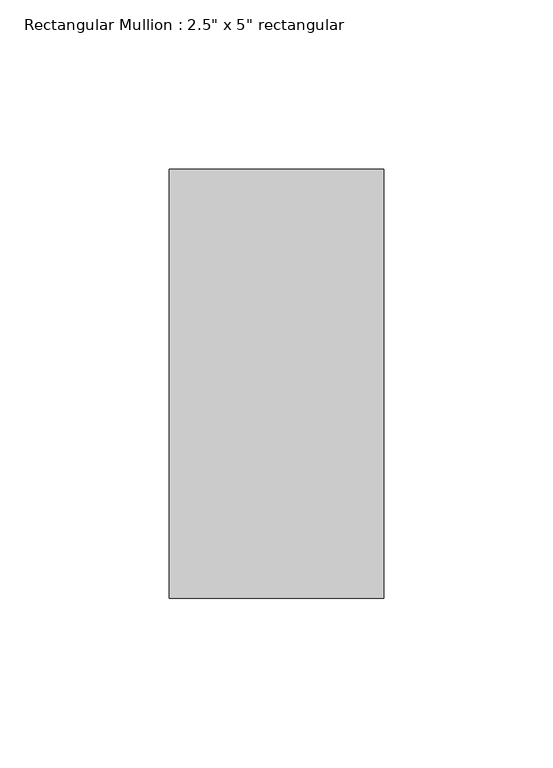
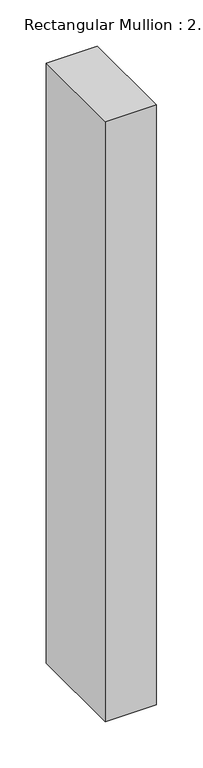
"""IFC4 building model written with IfcOpenShell, lengths in millimetres: member geometry."""

from ifc_helpers import new_model, si_unit, frame, origin, place, context, project, spatial, polyline, outline, extrude, source, transform, mapped, element, save


def member_c508cede(model_context):
    return source(origin(), model_context, "Body", "SweptSolid", [
        extrude(outline(polyline([(0.0, 63.5), (0.0, -63.5), (-63.5, -63.5), (-63.5, 63.5), (0.0, 63.5)])), frame((0.0, 0.0, -789.986197), z_axis=(0.0, 0.0, 1.0), x_axis=(1.0, 0.0, 0.0)), (0.0, 0.0, 1.0), 789.986197),
    ])


if __name__ == "__main__":
    model = new_model("IFC4")
    model_context = context("Model", 3, world=origin())
    ifc_project = project(units=[si_unit("LENGTHUNIT", "METRE", prefix="MILLI")], contexts=[model_context])
    site = spatial("IfcSite", under=ifc_project)
    building = spatial("IfcBuilding", under=site)
    placement = place(None, origin())
    member_shape = member_c508cede(model_context)
    element("IfcMember", 1, ObjectType="Rectangular Mullion : 2.5\" x 5\" rectangular", at=placement, inside=building, context=model_context, shape_type="MappedRepresentation", body=[
        mapped(member_shape, transform((0.0, 0.0, 0.0), x_axis=(1.0, 0.0, 0.0), y_axis=(0.0, 1.0, 0.0), z_axis=(0.0, 0.0, 1.0))),
    ])
    save(model, "model.ifc")

# Revit data of these elements
# Type "Rectangular Mullion : 2.5\" x 5\" rectangular"
#   built-in parameter 1007304 = 0.416667 (stored number, unit not read)
#   built-in parameter 1007301 = 0.104167 (stored number, unit not read)
#   built-in parameter 1007300 = 0.104167 (stored number, unit not read)
# Element 1 (IfcMember, "Rectangular Mullion : 2.5\" x 5\" rectangular")
#   Materials on its faces: "Aluminum"
# Materials
#   "Aluminum": class "Metal", colour RGB 247 247 247, transparency 0, Description = "Aluminum 6061", Cost = 0
